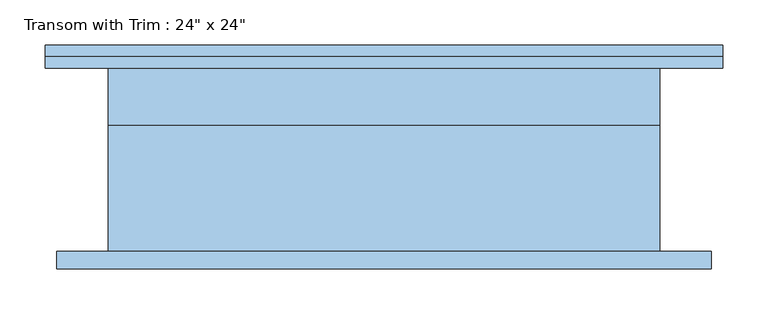
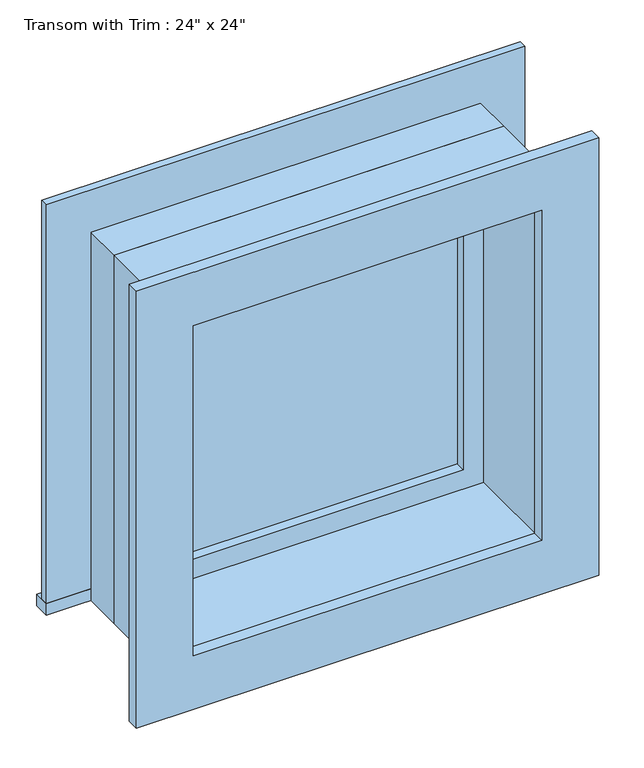
"""IFC4 building model written with IfcOpenShell, lengths in millimetres: window geometry."""

from ifc_helpers import new_model, si_unit, frame, origin, place, context, project, spatial, polyline, outline, extrude, source, transform, mapped, element, save


def window_e41d21a6(model_context):
    return source(origin(), model_context, "Body", "SweptSolid", [
        extrude(outline(polyline([(-412.75, 127.0), (336.55, 127.0), (336.55, 101.6), (-412.75, 101.6), (-412.75, 127.0)])), frame((0.0, 0.0, 2159.0), z_axis=(0.0, 0.0, 1.0), x_axis=(1.0, 0.0, 0.0)), (0.0, 0.0, 1.0), 19.05),
        extrude(outline(polyline([(2749.55, -323.85), (2749.55, 247.65), (2178.05, 247.65), (2178.05, 336.55), (2838.45, 336.55), (2838.45, -412.75), (2178.05, -412.75), (2178.05, -323.85), (2749.55, -323.85)])), frame((0.0, 101.6, 0.0), z_axis=(0.0, 1.0, 0.0), x_axis=(0.0, 0.0, 1.0)), (0.0, 0.0, 1.0), 12.7),
        extrude(outline(polyline([(2825.75, 323.85), (2825.75, -400.05), (2101.85, -400.05), (2101.85, 323.85), (2825.75, 323.85)]), holes=[polyline([(2736.85, 234.95), (2190.75, 234.95), (2190.75, -311.15), (2736.85, -311.15), (2736.85, 234.95)])]), frame((0.0, -120.65, 0.0), z_axis=(0.0, 1.0, 0.0), x_axis=(0.0, 0.0, 1.0)), (0.0, 0.0, 1.0), 19.05),
        extrude(outline(polyline([(203.2, 53.975), (-279.4, 53.975), (-279.4, 66.675), (203.2, 66.675), (203.2, 53.975)])), frame((0.0, 0.0, 2222.5), z_axis=(0.0, 0.0, 1.0), x_axis=(1.0, 0.0, 0.0)), (0.0, 0.0, 1.0), 482.6),
        extrude(outline(polyline([(2749.55, -323.85), (2178.05, -323.85), (2178.05, 247.65), (2749.55, 247.65), (2749.55, -323.85)]), holes=[polyline([(2705.1, -279.4), (2705.1, 203.2), (2222.5, 203.2), (2222.5, -279.4), (2705.1, -279.4)])]), frame((0.0, 38.1, 0.0), z_axis=(0.0, 1.0, 0.0), x_axis=(0.0, 0.0, 1.0)), (0.0, 0.0, 1.0), 44.45),
        extrude(outline(polyline([(2768.6, -342.9), (2159.0, -342.9), (2159.0, 266.7), (2768.6, 266.7), (2768.6, -342.9)]), holes=[polyline([(2736.85, -311.15), (2736.85, 234.95), (2190.75, 234.95), (2190.75, -311.15), (2736.85, -311.15)])]), frame((0.0, -101.6, 0.0), z_axis=(0.0, 1.0, 0.0), x_axis=(0.0, 0.0, 1.0)), (0.0, 0.0, 1.0), 139.7),
        extrude(outline(polyline([(2768.6, 266.7), (2768.6, -342.9), (2159.0, -342.9), (2159.0, 266.7), (2768.6, 266.7)]), holes=[polyline([(2749.55, 247.65), (2178.05, 247.65), (2178.05, -323.85), (2749.55, -323.85), (2749.55, 247.65)])]), frame((0.0, 38.1, 0.0), z_axis=(0.0, 1.0, 0.0), x_axis=(0.0, 0.0, 1.0)), (0.0, 0.0, 1.0), 63.5),
    ])


if __name__ == "__main__":
    model = new_model("IFC4")
    model_context = context("Model", 3, world=origin())
    ifc_project = project(units=[si_unit("LENGTHUNIT", "METRE", prefix="MILLI")], contexts=[model_context])
    site = spatial("IfcSite", under=ifc_project)
    building = spatial("IfcBuilding", under=site)
    placement = place(None, origin())
    window_shape = window_e41d21a6(model_context)
    element("IfcWindow", 1, ObjectType="Transom with Trim : 24\" x 24\"", at=placement, inside=building, context=model_context, shape_type="MappedRepresentation", body=[
        mapped(window_shape, transform((0.0, 0.0, 0.0), x_axis=(1.0, 0.0, 0.0), y_axis=(0.0, 1.0, 0.0), z_axis=(0.0, 0.0, 1.0))),
    ])
    save(model, "model.ifc")

# Revit data of these elements
# Type "Transom with Trim : 24\" x 24\""
#   Type Mark = "13"
#   Construction Type Id = "GSP4R"
#   Assembly Code = "B2020100"
#   Analytic Construction = "1/8 in Pilkington single glazing"
#   Visual Light Transmittance = 0.9
#   Solar Heat Gain Coefficient = 0.78
#   Heat Transfer Coefficient (U) = 0.6496 BTU/(h·ft²·°F)
#   Height = 2' - 0"
#   Default Sill Height = 7' - 1"
#   Trim Projection - Ext. = 0' - 0 1/2"
#   Trim Projection - Int. = 0' - 0 3/4"
#   Trim Width - Exterior = 0' - 3 1/2"
#   Trim Width - Interior = 0' - 3 1/2"
#   Width = 2' - 0"
#   Window Inset = 0' - 0 3/4"
#   Define Thermal Properties by = 1
#   Glass Pane Material = Glass
#   Sash Material = Sash
#   Trim Exterior Material = Trim
#   Trim Interior Material = Trim
#   Wall Closure = (empty or 0)
# Element 1 (IfcWindow, "Transom with Trim : 24\" x 24\"")
#   Materials on its faces: "Sash", "Trim", "Glass"
# Materials
#   "Glass": class "Glass", colour RGB 0 128 192, transparency 0.75, Description = "Soda Lime Glass", Cost = 0
#   "Sash": class "Wood", colour RGB 224 178 126, transparency 0
#   "Trim": class "Wood", colour RGB 224 178 126, transparency 0
